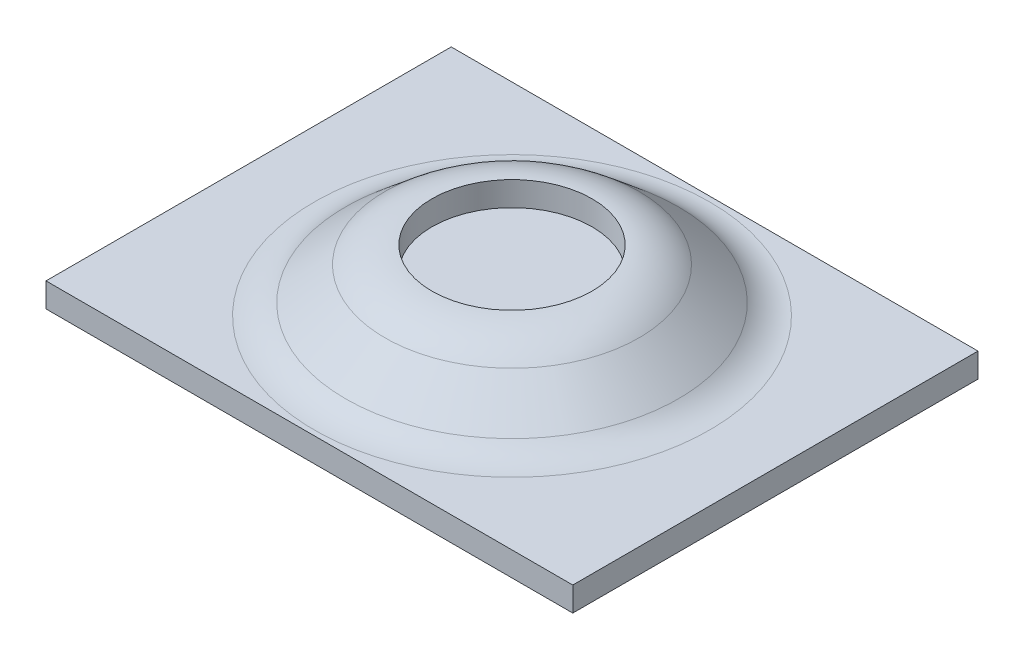
ISO-10303-21;
HEADER;
FILE_DESCRIPTION(('STEP AP214'),'2;1');
FILE_NAME('part.step','',(''),(''),'','','');
FILE_SCHEMA(('AUTOMOTIVE_DESIGN { 1 0 10303 214 1 1 1 1 }'));
ENDSEC;
DATA;
#1=APPLICATION_CONTEXT('core data for automotive mechanical design processes');
#2=APPLICATION_PROTOCOL_DEFINITION('international standard','automotive_design',2000,#1);
#3=PRODUCT_CONTEXT('',#1,'mechanical');
#4=PRODUCT('Part','Part','',(#3));
#5=PRODUCT_RELATED_PRODUCT_CATEGORY('part','',(#4));
#6=PRODUCT_DEFINITION_FORMATION('','',#4);
#7=PRODUCT_DEFINITION_CONTEXT('part definition',#1,'design');
#8=PRODUCT_DEFINITION('design','',#6,#7);
#9=PRODUCT_DEFINITION_SHAPE('','',#8);
#10=(LENGTH_UNIT() NAMED_UNIT(*) SI_UNIT(.MILLI.,.METRE.));
#11=(NAMED_UNIT(*) PLANE_ANGLE_UNIT() SI_UNIT($,.RADIAN.));
#12=(NAMED_UNIT(*) SI_UNIT($,.STERADIAN.) SOLID_ANGLE_UNIT());
#13=UNCERTAINTY_MEASURE_WITH_UNIT(LENGTH_MEASURE(1.E-05),#10,'distance_accuracy_value','');
#14=(GEOMETRIC_REPRESENTATION_CONTEXT(3) GLOBAL_UNCERTAINTY_ASSIGNED_CONTEXT((#13)) GLOBAL_UNIT_ASSIGNED_CONTEXT((#10,
#11,#12)) REPRESENTATION_CONTEXT('',''));
#15=CARTESIAN_POINT('',(0.,0.,0.));
#16=DIRECTION('',(0.,0.,1.));
#17=DIRECTION('',(1.,0.,0.));
#18=AXIS2_PLACEMENT_3D('',#15,#16,#17);
#19=CARTESIAN_POINT('',(0.,0.,0.));
#20=DIRECTION('',(0.,-1.,0.));
#21=DIRECTION('',(0.,0.,-1.));
#22=AXIS2_PLACEMENT_3D('',#19,#20,#21);
#23=PLANE('',#22);
#24=DIRECTION('',(0.,0.,1.));
#25=VECTOR('',#24,1.);
#26=CARTESIAN_POINT('',(-32.5,0.,25.));
#27=LINE('',#26,#25);
#28=CARTESIAN_POINT('',(-32.5,0.,-25.));
#29=VERTEX_POINT('',#28);
#30=CARTESIAN_POINT('',(-32.5,0.,25.));
#31=VERTEX_POINT('',#30);
#32=EDGE_CURVE('E82',#29,#31,#27,.T.);
#33=ORIENTED_EDGE('',*,*,#32,.F.);
#34=DIRECTION('',(1.,0.,0.));
#35=VECTOR('',#34,1.);
#36=CARTESIAN_POINT('',(0.,0.,-25.));
#37=LINE('',#36,#35);
#38=CARTESIAN_POINT('',(32.5,0.,-25.));
#39=VERTEX_POINT('',#38);
#40=EDGE_CURVE('E85',#29,#39,#37,.T.);
#41=ORIENTED_EDGE('',*,*,#40,.T.);
#42=DIRECTION('',(0.,0.,-1.));
#43=VECTOR('',#42,1.);
#44=CARTESIAN_POINT('',(32.5,0.,25.));
#45=LINE('',#44,#43);
#46=CARTESIAN_POINT('',(32.5,0.,25.));
#47=VERTEX_POINT('',#46);
#48=EDGE_CURVE('E64',#47,#39,#45,.T.);
#49=ORIENTED_EDGE('',*,*,#48,.F.);
#50=DIRECTION('',(-1.,0.,0.));
#51=VECTOR('',#50,1.);
#52=CARTESIAN_POINT('',(0.,0.,25.));
#53=LINE('',#52,#51);
#54=EDGE_CURVE('E86',#47,#31,#53,.T.);
#55=ORIENTED_EDGE('',*,*,#54,.T.);
#56=EDGE_LOOP('',(#33,#41,#49,#55));
#57=FACE_BOUND('',#56,.T.);
#58=ADVANCED_FACE('F42',(#57),#23,.T.);
#59=CARTESIAN_POINT('',(0.,3.,0.));
#60=DIRECTION('',(0.,-1.,0.));
#61=DIRECTION('',(0.,0.,-1.));
#62=AXIS2_PLACEMENT_3D('',#59,#60,#61);
#63=PLANE('',#62);
#64=CARTESIAN_POINT('',(0.,3.,0.));
#65=DIRECTION('',(0.,-1.,0.));
#66=DIRECTION('',(0.,0.,-1.));
#67=AXIS2_PLACEMENT_3D('',#64,#65,#66);
#68=CIRCLE('',#67,24.3842927362103);
#69=CARTESIAN_POINT('',(0.,3.,-24.3842927362103));
#70=VERTEX_POINT('',#69);
#71=EDGE_CURVE('E128',#70,#70,#68,.T.);
#72=ORIENTED_EDGE('',*,*,#71,.T.);
#73=EDGE_LOOP('',(#72));
#74=FACE_BOUND('',#73,.T.);
#75=DIRECTION('',(1.,0.,0.));
#76=VECTOR('',#75,1.);
#77=CARTESIAN_POINT('',(0.,3.,-25.));
#78=LINE('',#77,#76);
#79=CARTESIAN_POINT('',(-32.5,3.,-25.));
#80=VERTEX_POINT('',#79);
#81=CARTESIAN_POINT('',(32.5,3.,-25.));
#82=VERTEX_POINT('',#81);
#83=EDGE_CURVE('E52',#80,#82,#78,.T.);
#84=ORIENTED_EDGE('',*,*,#83,.F.);
#85=DIRECTION('',(0.,0.,1.));
#86=VECTOR('',#85,1.);
#87=CARTESIAN_POINT('',(-32.5,3.,25.));
#88=LINE('',#87,#86);
#89=CARTESIAN_POINT('',(-32.5,3.,25.));
#90=VERTEX_POINT('',#89);
#91=EDGE_CURVE('E80',#80,#90,#88,.T.);
#92=ORIENTED_EDGE('',*,*,#91,.T.);
#93=DIRECTION('',(-1.,0.,0.));
#94=VECTOR('',#93,1.);
#95=CARTESIAN_POINT('',(0.,3.,25.));
#96=LINE('',#95,#94);
#97=CARTESIAN_POINT('',(32.5,3.,25.));
#98=VERTEX_POINT('',#97);
#99=EDGE_CURVE('E12',#98,#90,#96,.T.);
#100=ORIENTED_EDGE('',*,*,#99,.F.);
#101=DIRECTION('',(0.,0.,-1.));
#102=VECTOR('',#101,1.);
#103=CARTESIAN_POINT('',(32.5,3.,25.));
#104=LINE('',#103,#102);
#105=EDGE_CURVE('E117',#98,#82,#104,.T.);
#106=ORIENTED_EDGE('',*,*,#105,.T.);
#107=EDGE_LOOP('',(#84,#92,#100,#106));
#108=FACE_BOUND('',#107,.T.);
#109=ADVANCED_FACE('F151',(#74,#108),#63,.F.);
#110=CARTESIAN_POINT('',(0.,9.,0.));
#111=DIRECTION('',(0.,-1.,0.));
#112=DIRECTION('',(0.,0.,-1.));
#113=AXIS2_PLACEMENT_3D('',#110,#111,#112);
#114=TOROIDAL_SURFACE('',#113,24.3842927362103,6.);
#115=ORIENTED_EDGE('',*,*,#71,.F.);
#116=EDGE_LOOP('',(#115));
#117=FACE_BOUND('',#116,.T.);
#118=CARTESIAN_POINT('',(0.,4.4037333412861,0.));
#119=DIRECTION('',(0.,-1.,0.));
#120=DIRECTION('',(0.,0.,-1.));
#121=AXIS2_PLACEMENT_3D('',#118,#119,#120);
#122=CIRCLE('',#121,20.5275670780911);
#123=CARTESIAN_POINT('',(0.,4.4037333412861,-20.5275670780911));
#124=VERTEX_POINT('',#123);
#125=EDGE_CURVE('E129',#124,#124,#122,.T.);
#126=ORIENTED_EDGE('',*,*,#125,.T.);
#127=EDGE_LOOP('',(#126));
#128=FACE_BOUND('',#127,.T.);
#129=ADVANCED_FACE('F160',(#117,#128),#114,.F.);
#130=CARTESIAN_POINT('',(0.,8.48422240332173,0.));
#131=DIRECTION('',(0.,-1.,0.));
#132=DIRECTION('',(0.,0.,-1.));
#133=AXIS2_PLACEMENT_3D('',#130,#131,#132);
#134=CONICAL_SURFACE('',#133,15.6646295788687,0.872664625997174);
#135=ORIENTED_EDGE('',*,*,#125,.F.);
#136=EDGE_LOOP('',(#135));
#137=FACE_BOUND('',#136,.T.);
#138=CARTESIAN_POINT('',(0.,8.48422240332173,0.));
#139=DIRECTION('',(0.,-1.,0.));
#140=DIRECTION('',(0.,0.,-1.));
#141=AXIS2_PLACEMENT_3D('',#138,#139,#140);
#142=CIRCLE('',#141,15.6646295788687);
#143=CARTESIAN_POINT('',(0.,8.48422240332173,-15.6646295788687));
#144=VERTEX_POINT('',#143);
#145=EDGE_CURVE('E124',#144,#144,#142,.T.);
#146=ORIENTED_EDGE('',*,*,#145,.T.);
#147=EDGE_LOOP('',(#146));
#148=FACE_BOUND('',#147,.T.);
#149=ADVANCED_FACE('F194',(#137,#148),#134,.T.);
#150=CARTESIAN_POINT('',(0.,1.58982241525087,0.));
#151=DIRECTION('',(0.,-1.,0.));
#152=DIRECTION('',(0.,0.,-1.));
#153=AXIS2_PLACEMENT_3D('',#150,#151,#152);
#154=TOROIDAL_SURFACE('',#153,9.87954109168991,9.);
#155=CARTESIAN_POINT('',(0.,10.5898224152509,0.));
#156=DIRECTION('',(0.,1.,0.));
#157=DIRECTION('',(0.,0.,1.));
#158=AXIS2_PLACEMENT_3D('',#155,#156,#157);
#159=CIRCLE('',#158,9.87954109168991);
#160=CARTESIAN_POINT('',(0.,10.5898224152509,9.87954109168991));
#161=VERTEX_POINT('',#160);
#162=EDGE_CURVE('E115',#161,#161,#159,.T.);
#163=ORIENTED_EDGE('',*,*,#162,.F.);
#164=EDGE_LOOP('',(#163));
#165=FACE_BOUND('',#164,.T.);
#166=ORIENTED_EDGE('',*,*,#145,.F.);
#167=EDGE_LOOP('',(#166));
#168=FACE_BOUND('',#167,.T.);
#169=ADVANCED_FACE('F146',(#165,#168),#154,.T.);
#170=CARTESIAN_POINT('',(-32.5,-7.,-25.));
#171=DIRECTION('',(0.,0.,-1.));
#172=DIRECTION('',(-1.,0.,0.));
#173=AXIS2_PLACEMENT_3D('',#170,#171,#172);
#174=PLANE('',#173);
#175=ORIENTED_EDGE('',*,*,#40,.F.);
#176=DIRECTION('',(0.,1.,0.));
#177=VECTOR('',#176,1.);
#178=CARTESIAN_POINT('',(-32.5,0.,-25.));
#179=LINE('',#178,#177);
#180=EDGE_CURVE('E97',#29,#80,#179,.T.);
#181=ORIENTED_EDGE('',*,*,#180,.T.);
#182=ORIENTED_EDGE('',*,*,#83,.T.);
#183=DIRECTION('',(0.,1.,0.));
#184=VECTOR('',#183,1.);
#185=CARTESIAN_POINT('',(32.5,0.,-25.));
#186=LINE('',#185,#184);
#187=EDGE_CURVE('E100',#39,#82,#186,.T.);
#188=ORIENTED_EDGE('',*,*,#187,.F.);
#189=EDGE_LOOP('',(#175,#181,#182,#188));
#190=FACE_BOUND('',#189,.T.);
#191=ADVANCED_FACE('F94',(#190),#174,.T.);
#192=CARTESIAN_POINT('',(-32.5,-7.,25.));
#193=DIRECTION('',(0.,0.,1.));
#194=DIRECTION('',(1.,0.,0.));
#195=AXIS2_PLACEMENT_3D('',#192,#193,#194);
#196=PLANE('',#195);
#197=ORIENTED_EDGE('',*,*,#99,.T.);
#198=DIRECTION('',(0.,1.,0.));
#199=VECTOR('',#198,1.);
#200=CARTESIAN_POINT('',(-32.5,0.,25.));
#201=LINE('',#200,#199);
#202=EDGE_CURVE('E105',#31,#90,#201,.T.);
#203=ORIENTED_EDGE('',*,*,#202,.F.);
#204=ORIENTED_EDGE('',*,*,#54,.F.);
#205=DIRECTION('',(0.,1.,0.));
#206=VECTOR('',#205,1.);
#207=CARTESIAN_POINT('',(32.5,0.,25.));
#208=LINE('',#207,#206);
#209=EDGE_CURVE('E104',#47,#98,#208,.T.);
#210=ORIENTED_EDGE('',*,*,#209,.T.);
#211=EDGE_LOOP('',(#197,#203,#204,#210));
#212=FACE_BOUND('',#211,.T.);
#213=ADVANCED_FACE('F138',(#212),#196,.T.);
#214=CARTESIAN_POINT('',(-32.5,0.,25.));
#215=DIRECTION('',(-1.,0.,0.));
#216=DIRECTION('',(0.,0.,1.));
#217=AXIS2_PLACEMENT_3D('',#214,#215,#216);
#218=PLANE('',#217);
#219=ORIENTED_EDGE('',*,*,#91,.F.);
#220=ORIENTED_EDGE('',*,*,#180,.F.);
#221=ORIENTED_EDGE('',*,*,#32,.T.);
#222=ORIENTED_EDGE('',*,*,#202,.T.);
#223=EDGE_LOOP('',(#219,#220,#221,#222));
#224=FACE_BOUND('',#223,.T.);
#225=ADVANCED_FACE('F103',(#224),#218,.T.);
#226=CARTESIAN_POINT('',(32.5,0.,25.));
#227=DIRECTION('',(1.,0.,0.));
#228=DIRECTION('',(0.,0.,-1.));
#229=AXIS2_PLACEMENT_3D('',#226,#227,#228);
#230=PLANE('',#229);
#231=ORIENTED_EDGE('',*,*,#48,.T.);
#232=ORIENTED_EDGE('',*,*,#187,.T.);
#233=ORIENTED_EDGE('',*,*,#105,.F.);
#234=ORIENTED_EDGE('',*,*,#209,.F.);
#235=EDGE_LOOP('',(#231,#232,#233,#234));
#236=FACE_BOUND('',#235,.T.);
#237=ADVANCED_FACE('F135',(#236),#230,.T.);
#238=CARTESIAN_POINT('',(0.,-12.4101775847491,0.));
#239=DIRECTION('',(0.,1.,0.));
#240=DIRECTION('',(0.,0.,1.));
#241=AXIS2_PLACEMENT_3D('',#238,#239,#240);
#242=CYLINDRICAL_SURFACE('',#241,9.87954109168991);
#243=ORIENTED_EDGE('',*,*,#162,.T.);
#244=EDGE_LOOP('',(#243));
#245=FACE_BOUND('',#244,.T.);
#246=CARTESIAN_POINT('',(0.,7.58982241525087,0.));
#247=DIRECTION('',(0.,-1.,0.));
#248=DIRECTION('',(0.,0.,-1.));
#249=AXIS2_PLACEMENT_3D('',#246,#247,#248);
#250=CIRCLE('',#249,9.87954109168991);
#251=CARTESIAN_POINT('',(0.,7.58982241525087,-9.87954109168991));
#252=VERTEX_POINT('',#251);
#253=EDGE_CURVE('E114',#252,#252,#250,.F.);
#254=ORIENTED_EDGE('',*,*,#253,.F.);
#255=EDGE_LOOP('',(#254));
#256=FACE_BOUND('',#255,.T.);
#257=ADVANCED_FACE('F175',(#245,#256),#242,.F.);
#258=CARTESIAN_POINT('',(0.,1.58982241525087,0.));
#259=DIRECTION('',(0.,-1.,0.));
#260=DIRECTION('',(0.,0.,-1.));
#261=AXIS2_PLACEMENT_3D('',#258,#259,#260);
#262=TOROIDAL_SURFACE('',#261,9.87954109168991,6.);
#263=ORIENTED_EDGE('',*,*,#253,.T.);
#264=EDGE_LOOP('',(#263));
#265=FACE_BOUND('',#264,.T.);
#266=CARTESIAN_POINT('',(0.,6.18608907396477,0.));
#267=DIRECTION('',(0.,-1.,0.));
#268=DIRECTION('',(0.,0.,-1.));
#269=AXIS2_PLACEMENT_3D('',#266,#267,#268);
#270=CIRCLE('',#269,13.7362667498091);
#271=CARTESIAN_POINT('',(0.,6.18608907396477,-13.7362667498091));
#272=VERTEX_POINT('',#271);
#273=EDGE_CURVE('E132',#272,#272,#270,.T.);
#274=ORIENTED_EDGE('',*,*,#273,.T.);
#275=EDGE_LOOP('',(#274));
#276=FACE_BOUND('',#275,.T.);
#277=ADVANCED_FACE('F46',(#265,#276),#262,.F.);
#278=CARTESIAN_POINT('',(0.,6.18608907396477,0.));
#279=DIRECTION('',(0.,-1.,0.));
#280=DIRECTION('',(0.,0.,-1.));
#281=AXIS2_PLACEMENT_3D('',#278,#279,#280);
#282=CONICAL_SURFACE('',#281,13.7362667498091,0.872664625997173);
#283=ORIENTED_EDGE('',*,*,#273,.F.);
#284=EDGE_LOOP('',(#283));
#285=FACE_BOUND('',#284,.T.);
#286=CARTESIAN_POINT('',(0.,3.,0.));
#287=DIRECTION('',(0.,-1.,0.));
#288=DIRECTION('',(0.,0.,-1.));
#289=AXIS2_PLACEMENT_3D('',#286,#287,#288);
#290=CIRCLE('',#289,17.5332998500318);
#291=CARTESIAN_POINT('',(0.,3.,-17.5332998500318));
#292=VERTEX_POINT('',#291);
#293=EDGE_CURVE('E107',#292,#292,#290,.T.);
#294=ORIENTED_EDGE('',*,*,#293,.T.);
#295=EDGE_LOOP('',(#294));
#296=FACE_BOUND('',#295,.T.);
#297=ADVANCED_FACE('F163',(#285,#296),#282,.F.);
#298=CARTESIAN_POINT('',(0.,3.,0.));
#299=DIRECTION('',(0.,-1.,0.));
#300=DIRECTION('',(0.,0.,-1.));
#301=AXIS2_PLACEMENT_3D('',#298,#299,#300);
#302=PLANE('',#301);
#303=ORIENTED_EDGE('',*,*,#293,.F.);
#304=EDGE_LOOP('',(#303));
#305=FACE_BOUND('',#304,.T.);
#306=ADVANCED_FACE('F161',(#305),#302,.F.);
#307=CLOSED_SHELL('',(#58,#109,#129,#149,#169,#191,#213,#225,#237,#257,#277,#297,#306));
#308=MANIFOLD_SOLID_BREP('B2',#307);
#309=ADVANCED_BREP_SHAPE_REPRESENTATION('',(#18,#308),#14);
#310=SHAPE_DEFINITION_REPRESENTATION(#9,#309);
ENDSEC;
END-ISO-10303-21;
